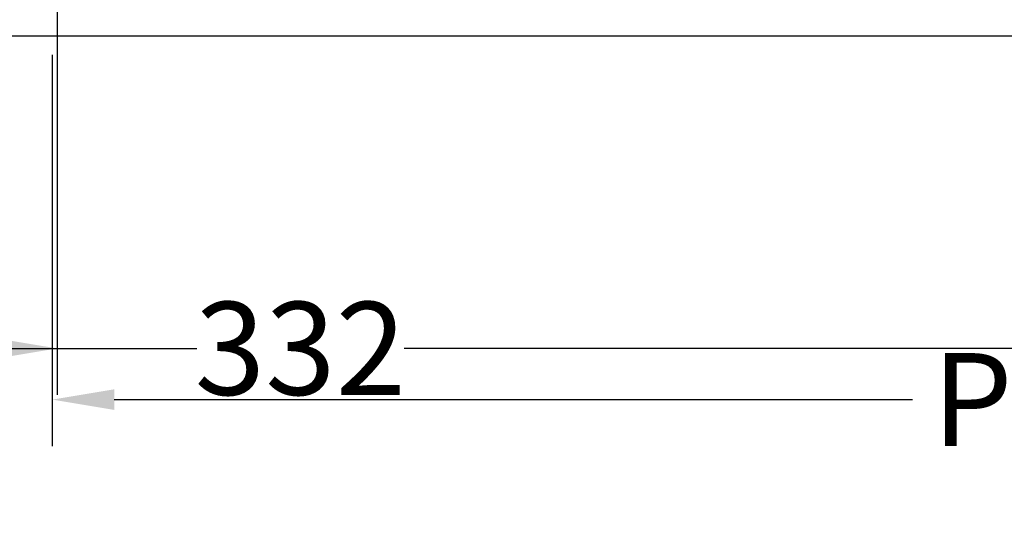
# Model space of a CAD drawing. Units: inches. Extents: x 89 to 490, y -59 to 378.
# Tile 2 of 20: x 275 to 339, y -59 to -26. Entities that reach past the tile are written whole.
import ezdxf

# ---------------------------------------------------------------- set-up
doc = ezdxf.new("R2010")
doc.units = ezdxf.units.IN
doc.header["$MEASUREMENT"] = 0
doc.layers.add('A-ANNO-DIMS', color=2, linetype='Continuous', lineweight=18)
doc.layers.add('L-PLNT-EDGE', color=31, linetype='Continuous', lineweight=25)
doc.styles.get("Standard").update_dxf_attribs({"font": 'arial.ttf'})
doc.dimstyles.get("Standard").update_dxf_attribs({"dimtxt": 6, "dimasz": 4, "dimexe": 3, "dimexo": 3, "dimgap": 0.09, "dimtad": 0, "dimtih": 1, "dimtoh": 1, "dimdec": 1, "dimzin": 0, "dimdsep": 46, "dimlunit": 3, "dimtxsty": 'Standard', "dimcen": 0.09, "dimadec": 0, "dimazin": 0, "dimtfac": 1, "dimtdec": 1, "dimtofl": 0, "dimtmove": 0, "dimatfit": 3, "dimfxl": 1, "dimtolj": 1, "dimtzin": 0, "dimarcsym": 0})

# ---------------------------------------------------------------- blocks, each defined once
blk = doc.blocks.new('*D46')
at = {"layer": 'A-ANNO-DIMS', "color": 0, "lineweight": -2, "transparency": 16777216}
for p, q in [((277.443, -27.866), (277.443, -53.11)), ((445.739, -27.866), (445.739, -53.11)), ((281.443, -50.11), (332.892, -50.11)), ((441.739, -50.11), (390.289, -50.11))]:
    blk.add_line(p, q, dxfattribs=at)
at = {"layer": 'A-ANNO-DIMS', "color": 0, "transparency": 16777216}
for points in [[(281.443, -49.443), (281.443, -50.777), (277.443, -50.11)], [(441.739, -49.443), (441.739, -50.777), (445.739, -50.11)]]:
    blk.add_solid(points, dxfattribs=at)
at = {"layer": 'Defpoints', "color": 0, "transparency": 16777216}
for p in [(277.443, -24.866), (445.739, -24.866), (445.739, -50.11)]:
    blk.add_point(p, dxfattribs=at)
at = {"layer": 'A-ANNO-DIMS', "color": 0, "transparency": 16777216, "insert": (361.591, -50.11), "char_height": 6, "attachment_point": 5}
blk.add_mtext('\\A1;PLANTING 168', dxfattribs=at)
blk = doc.blocks.new('*D48')
at = {"layer": 'A-ANNO-DIMS', "color": 0, "lineweight": -2, "transparency": 16777216}
for p, q in [((127.441, 10.741), (127.441, -49.809)), ((459.441, -29.659), (459.441, -49.809)), ((131.441, -46.809), (286.756, -46.809)), ((455.441, -46.809), (300.127, -46.809))]:
    blk.add_line(p, q, dxfattribs=at)
at = {"layer": 'A-ANNO-DIMS', "color": 0, "transparency": 16777216}
for points in [[(131.441, -46.143), (131.441, -47.476), (127.441, -46.809)], [(455.441, -46.143), (455.441, -47.476), (459.441, -46.809)]]:
    blk.add_solid(points, dxfattribs=at)
at = {"layer": 'Defpoints', "color": 0, "transparency": 16777216}
for p in [(127.441, 13.741), (459.441, -26.659), (459.441, -46.809)]:
    blk.add_point(p, dxfattribs=at)
at = {"layer": 'A-ANNO-DIMS', "color": 0, "transparency": 16777216, "insert": (293.441, -46.809), "char_height": 6, "attachment_point": 5}
blk.add_mtext('\\A1;332', dxfattribs=at)
blk = doc.blocks.new('*D74')
at = {"layer": 'A-ANNO-DIMS', "color": 0, "lineweight": -2, "transparency": 16777216}
for p, q in [((249.441, 341.741), (249.441, -49.809)), ((277.753, 341.347), (277.753, -49.809)), ((253.441, -46.809), (253.912, -46.809)), ((273.753, -46.809), (273.283, -46.809))]:
    blk.add_line(p, q, dxfattribs=at)
at = {"layer": 'A-ANNO-DIMS', "color": 0, "transparency": 16777216}
for points in [[(253.441, -46.143), (253.441, -47.476), (249.441, -46.809)], [(273.753, -46.143), (273.753, -47.476), (277.753, -46.809)]]:
    blk.add_solid(points, dxfattribs=at)
at = {"layer": 'Defpoints', "color": 0, "transparency": 16777216}
for p in [(249.441, 344.741), (277.753, 344.347), (277.753, -46.809)]:
    blk.add_point(p, dxfattribs=at)
at = {"layer": 'A-ANNO-DIMS', "color": 0, "transparency": 16777216, "insert": (263.597, -46.809), "char_height": 6, "attachment_point": 5}
blk.add_mtext('\\A1;28.31', dxfattribs=at)

msp = doc.modelspace()

# ---------------------------------------------------------------- linework, layer by layer
at = {"layer": 'L-PLNT-EDGE'}
msp.add_line((459.4414, -26.6594), (265.4414, -26.6594), dxfattribs=at)

# ---------------------------------------------------------------- dimensions: what is measured, and where the dimension line sits
at = {"layer": 'A-ANNO-DIMS'}
for base, p1, p2, override, picture, middle in [((277.7535, -46.8094), (249.4414, 344.7413), (277.7535, 344.3468), {"dimdec": 2, "dimlfac": 1, "dimrnd": 0, "dimzin": 0, "dimdsep": 46, "dimlunit": 2}, '*D74', (263.5974, -46.8094)), ((459.4414, -46.8094), (127.4414, 13.7413), (459.4414, -26.6594), {"dimdec": 0, "dimlfac": 1, "dimrnd": 0, "dimzin": 0, "dimdsep": 46, "dimlunit": 2}, '*D48', (293.4414, -46.8094))]:
    dim = msp.add_linear_dim(base=base, p1=p1, p2=p2, dimstyle='Standard', override=override, dxfattribs=at)
    dim.commit()
    dim.dimension.update_dxf_attribs({"geometry": picture, "text_midpoint": middle})
dim = msp.add_linear_dim(base=(445.7386, -50.11), p1=(277.443, -24.8656), p2=(445.7386, -24.8656), text='PLANTING <>', dimstyle='Standard', override={"dimdec": 0, "dimlfac": 1, "dimrnd": 0, "dimzin": 0, "dimdsep": 46, "dimlunit": 2}, dxfattribs=at)
dim.commit()
dim.dimension.update_dxf_attribs({"geometry": '*D46', "text_midpoint": (361.5908, -50.11)})

doc.saveas('drawing.dxf')
